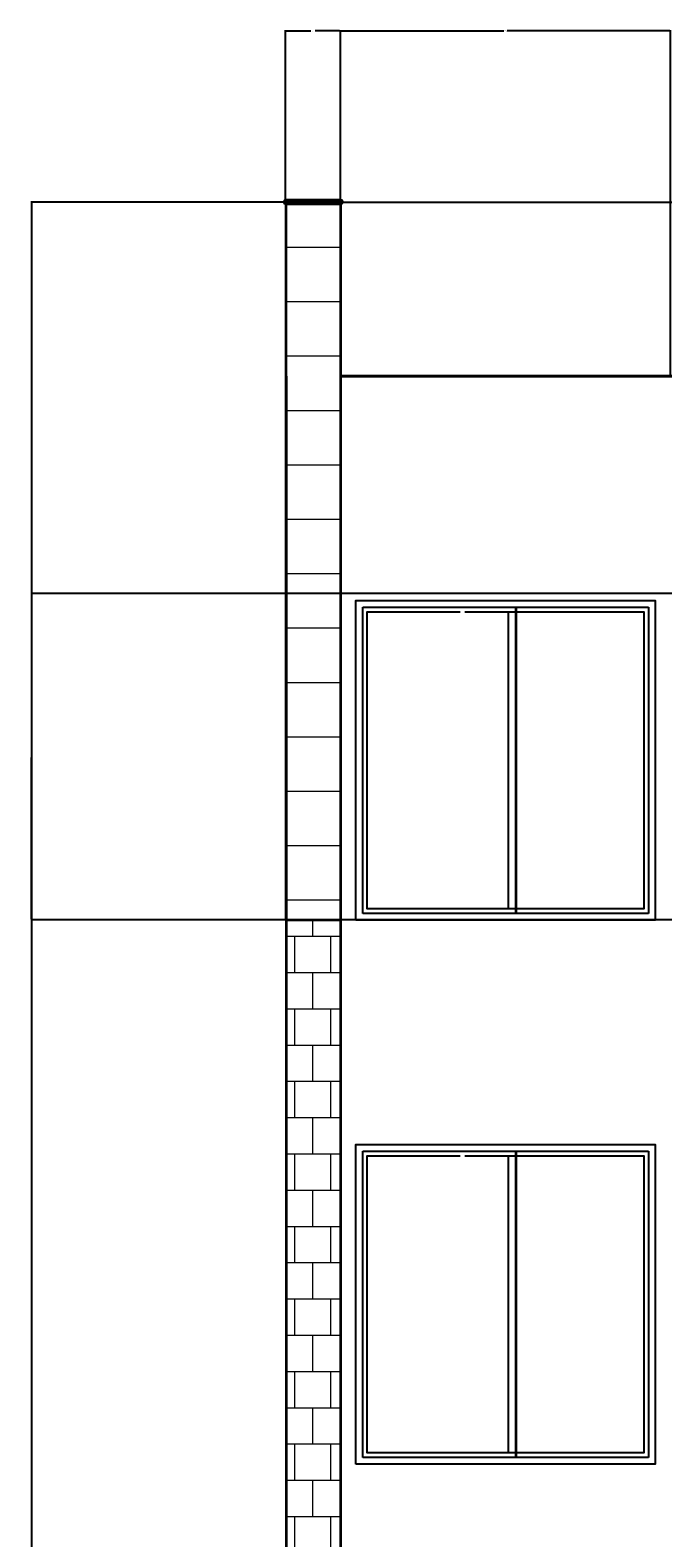
# Model space of a CAD drawing. Units: inches. Extents: x 10 to 404, y -77 to 696.
# Tile 4 of 5: x 10 to 149, y 363 to 696. Entities that reach past the tile are written whole.
import ezdxf

# ---------------------------------------------------------------- set-up
doc = ezdxf.new("R2010")
doc.units = ezdxf.units.IN
doc.header["$MEASUREMENT"] = 0
for name, color, linetype, lineweight in [('A-ANNO-DIMS', 2, 'Continuous', 18), ('A-ELEV', 7, 'Continuous', 35), ('A-ELEV-PATT', 8, 'Continuous', 13), ('A-GLAZ', 4, 'Continuous', 25)]:
    doc.layers.add(name, color=color, linetype=linetype, lineweight=lineweight)
doc.styles.get("Standard").update_dxf_attribs({"font": 'arial.ttf'})
doc.dimstyles.get("Standard").update_dxf_attribs({"dimtxt": 0.18, "dimasz": 0.18, "dimexe": 0.18, "dimexo": 0.0625, "dimgap": 0.09, "dimtad": 0, "dimtih": 1, "dimtoh": 1, "dimdec": 4, "dimzin": 0, "dimdsep": 46, "dimtxsty": 'Standard', "dimcen": 0.09, "dimadec": 0, "dimazin": 0, "dimtfac": 1, "dimtdec": 4, "dimtofl": 0, "dimtmove": 0, "dimatfit": 3, "dimfxl": 1, "dimtolj": 1, "dimtzin": 0, "dimarcsym": 0})

# ---------------------------------------------------------------- blocks, each defined once
blk = doc.blocks.new('WIN-SLIDING-2P')
for p, q in [((83.01, 21.05), (83.01, 88.58)), ((83.01, 88.58), (105.51, 88.58)), ((105.51, 88.58), (146.03, 88.58)), ((146.03, 88.58), (146.03, 21.05)), ((105.51, 21.05), (83.01, 21.05)), ((146.03, 21.05), (105.51, 21.05))]:
    blk.add_line(p, q)
blk.add_lwpolyline([(81.51, 19.55), (81.51, 90.08), (147.53, 90.08), (147.53, 19.55)], close=True)
blk.add_lwpolyline([(115.07, 87.58), (115.07, 22.05), (84.01, 22.05), (84.01, 87.58), (104.51, 87.58)])
blk = doc.blocks.new('*D10')
at = {"layer": 'A-ANNO-DIMS', "color": 0, "lineweight": -2, "transparency": 16777216}
for p, q in [((65.94, 657.96), (9.76, 657.96)), ((9.94, 657.78), (9.94, 315.77)), ((9.94, -26.6), (9.94, 315.41)), ((176.46, -26.78), (9.76, -26.78))]:
    blk.add_line(p, q, dxfattribs=at)
at = {"layer": 'A-ANNO-DIMS', "color": 0, "transparency": 16777216}
for points in [[(9.91, 657.78), (9.97, 657.78), (9.94, 657.96)], [(9.91, -26.6), (9.97, -26.6), (9.94, -26.78)]]:
    blk.add_solid(points, dxfattribs=at)
at = {"layer": 'Defpoints', "color": 0, "transparency": 16777216}
for p in [(9.94, 657.96), (66.01, 657.96), (176.53, -26.78)]:
    blk.add_point(p, dxfattribs=at)
at = {"layer": 'A-ANNO-DIMS', "color": 0, "transparency": 16777216, "insert": (9.94, 315.59), "char_height": 0.18, "attachment_point": 5}
blk.add_mtext('\\A1;684.7', dxfattribs=at)
blk = doc.blocks.new('*D17')
at = {"layer": 'A-ANNO-DIMS', "color": 0, "lineweight": -2, "transparency": 16777216}
for p, q in [((66.01, 658.02), (66.01, 695.87)), ((66.19, 695.69), (71.6, 695.69)), ((77.92, 695.69), (72.51, 695.69)), ((78.1, 657.66), (78.1, 695.87))]:
    blk.add_line(p, q, dxfattribs=at)
at = {"layer": 'A-ANNO-DIMS', "color": 0, "transparency": 16777216}
for points in [[(66.19, 695.72), (66.19, 695.66), (66.01, 695.69)], [(77.92, 695.72), (77.92, 695.66), (78.1, 695.69)]]:
    blk.add_solid(points, dxfattribs=at)
at = {"layer": 'Defpoints', "color": 0, "transparency": 16777216}
for p in [(78.1, 695.69), (66.01, 657.96), (78.1, 657.59)]:
    blk.add_point(p, dxfattribs=at)
at = {"layer": 'A-ANNO-DIMS', "color": 0, "transparency": 16777216, "insert": (72.05, 695.69), "char_height": 0.18, "attachment_point": 5}
blk.add_mtext('\\A1;12.095', dxfattribs=at)
blk = doc.blocks.new('*D18')
at = {"layer": 'A-ANNO-DIMS', "color": 0, "lineweight": -2, "transparency": 16777216}
for p, q in [((78.1, 619.62), (78.1, 695.87)), ((78.28, 695.69), (114.12, 695.69)), ((150.75, 695.69), (114.91, 695.69)), ((150.93, 619.62), (150.93, 695.87))]:
    blk.add_line(p, q, dxfattribs=at)
at = {"layer": 'A-ANNO-DIMS', "color": 0, "transparency": 16777216}
for points in [[(78.28, 695.72), (78.28, 695.66), (78.1, 695.69)], [(150.75, 695.72), (150.75, 695.66), (150.93, 695.69)]]:
    blk.add_solid(points, dxfattribs=at)
at = {"layer": 'Defpoints', "color": 0, "transparency": 16777216}
for p in [(150.93, 695.69), (78.1, 619.55), (150.93, 619.55)]:
    blk.add_point(p, dxfattribs=at)
at = {"layer": 'A-ANNO-DIMS', "color": 0, "transparency": 16777216, "insert": (114.52, 695.69), "char_height": 0.18, "attachment_point": 5}
blk.add_mtext('\\A1;72.83', dxfattribs=at)
blk = doc.blocks.new('*D35')
at = {"layer": 'A-ANNO-DIMS', "color": 0, "lineweight": -2, "transparency": 16777216}
for p, q in [((66.07, 657.96), (403.47, 657.96)), ((403.29, 657.78), (403.29, 638.94)), ((403.29, 619.73), (403.29, 638.58)), ((354.63, 619.55), (403.47, 619.55))]:
    blk.add_line(p, q, dxfattribs=at)
at = {"layer": 'A-ANNO-DIMS', "color": 0, "transparency": 16777216}
for points in [[(403.26, 657.78), (403.32, 657.78), (403.29, 657.96)], [(403.26, 619.73), (403.32, 619.73), (403.29, 619.55)]]:
    blk.add_solid(points, dxfattribs=at)
at = {"layer": 'Defpoints', "color": 0, "transparency": 16777216}
for p in [(66.01, 657.96), (403.29, 657.96), (354.56, 619.55)]:
    blk.add_point(p, dxfattribs=at)
at = {"layer": 'A-ANNO-DIMS', "color": 0, "transparency": 16777216, "insert": (403.29, 638.76), "char_height": 0.18, "attachment_point": 5}
blk.add_mtext('\\A1;38.41', dxfattribs=at)
blk = doc.blocks.new('*D71')
at = {"layer": 'A-ANNO-DIMS', "color": 0, "lineweight": -2, "transparency": 16777216}
for p, q in [((203.6, 571.6), (9.76, 571.6)), ((9.94, 571.42), (9.94, 535.78)), ((9.94, 499.78), (9.94, 535.42)), ((203.6, 499.6), (9.76, 499.6))]:
    blk.add_line(p, q, dxfattribs=at)
at = {"layer": 'A-ANNO-DIMS', "color": 0, "transparency": 16777216}
for points in [[(9.91, 571.42), (9.97, 571.42), (9.94, 571.6)], [(9.91, 499.78), (9.97, 499.78), (9.94, 499.6)]]:
    blk.add_solid(points, dxfattribs=at)
at = {"layer": 'Defpoints', "color": 0, "transparency": 16777216}
for p in [(9.94, 571.6), (203.67, 571.6), (203.67, 499.6)]:
    blk.add_point(p, dxfattribs=at)
at = {"layer": 'A-ANNO-DIMS', "color": 0, "transparency": 16777216, "insert": (9.94, 535.6), "char_height": 0.18, "attachment_point": 5}
blk.add_mtext('\\A1;72', dxfattribs=at)

msp = doc.modelspace()

# ---------------------------------------------------------------- hatches: boundary and pattern name
at = {"layer": 'A-ELEV-PATT'}
h = msp.add_hatch(dxfattribs=at)
h.set_pattern_fill('_USER', color=256, scale=12, pattern_type=0)
h.set_pattern_definition([(0, (0, 0), (0, 12), [])])
h.paths.add_polyline_path([(78.1013, 657.5934), (66.1013, 657.5934), (66.1013, 499.5535), (78.1013, 499.5535)])
h = msp.add_hatch(dxfattribs=at)
h.set_pattern_fill('AR-B88', color=256)
h.paths.add_polyline_path([(78.1013, 499.5535), (66.1013, 499.5535), (66.1013, 19.5535), (78.1013, 19.5535)])

# ---------------------------------------------------------------- linework, layer by layer
at = {"layer": 'A-ELEV'}
for p, q in [((78.1965, 658.3411), (66.0062, 658.3411)), ((66.1013, 619.5535), (66.1013, 19.5535)), ((341.8668, 619.5535), (78.1013, 619.5535)), ((78.1013, 619.5535), (341.8668, 619.5535)), ((78.1013, 619.5535), (78.1013, 19.5535)), ((116.8527, 501.0535), (116.8527, 568.5811)), ((116.8527, 381.0535), (116.8527, 448.5811))]:
    msp.add_line(p, q, dxfattribs=at)
msp.add_lwpolyline([(78.1013, 499.5535), (66.1013, 499.5535), (66.1013, 657.5934), (78.1013, 657.5934)], close=True, dxfattribs=at)
for centre, start, end in [((66.0062, 657.9612), 90, 284.503141), ((78.1965, 657.9612), 255.496859, 90)]:
    msp.add_arc(centre, 0.3799, start, end, dxfattribs=at)
at = {"layer": 'A-GLAZ'}
for points in [[(105.5054, 567.5811), (145.0304, 567.5811), (145.0304, 502.0535), (105.5054, 502.0535)], [(105.5054, 447.5811), (145.0304, 447.5811), (145.0304, 382.0535), (105.5054, 382.0535)]]:
    msp.add_lwpolyline(points, dxfattribs=at)

# ---------------------------------------------------------------- block references
for p in [(0, 480), (0, 360)]:
    msp.add_blockref('WIN-SLIDING-2P', p, dxfattribs=at)

# ---------------------------------------------------------------- dimensions: what is measured, and where the dimension line sits
at = {"layer": 'A-ANNO-DIMS'}
for base, p1, p2, override, picture, middle in [((78.1013, 695.6911), (66.0062, 657.9612), (78.1013, 657.5934), {"dimdec": 3, "dimlfac": 1, "dimrnd": 0, "dimzin": 0, "dimdsep": 46, "dimlunit": 2}, '*D17', (72.0538, 695.6911)), ((150.9344, 695.6911), (78.1013, 619.5535), (150.9344, 619.5535), {"dimdec": 2, "dimlfac": 1, "dimrnd": 0, "dimzin": 0, "dimdsep": 46, "dimlunit": 2}, '*D18', (114.5179, 695.6911))]:
    dim = msp.add_linear_dim(base=base, p1=p1, p2=p2, dimstyle='Standard', override=override, dxfattribs=at)
    dim.commit()
    dim.dimension.update_dxf_attribs({"geometry": picture, "text_midpoint": middle})
for base, p1, p2, override, picture, middle in [((9.9405, 657.9612), (176.5266, -26.7816), (66.0062, 657.9612), {"dimdec": 1, "dimlfac": 1, "dimrnd": 0, "dimzin": 0, "dimdsep": 46, "dimlunit": 2}, '*D10', (9.9405, 315.5898)), ((403.2856, 657.9612), (354.5631, 619.5535), (66.0062, 657.9612), {"dimdec": 2, "dimlfac": 1, "dimrnd": 0, "dimzin": 0, "dimdsep": 46, "dimlunit": 2}, '*D35', (403.2856, 638.7574)), ((9.9405, 571.6046), (203.6671, 499.6046), (203.6671, 571.6046), {"dimdec": 0, "dimlfac": 1, "dimrnd": 0, "dimzin": 0, "dimdsep": 46, "dimlunit": 2}, '*D71', (9.9405, 535.6046))]:
    dim = msp.add_linear_dim(base=base, p1=p1, p2=p2, angle=90, dimstyle='Standard', override=override, dxfattribs=at)
    dim.commit()
    dim.dimension.update_dxf_attribs({"geometry": picture, "text_midpoint": middle})

doc.saveas('drawing.dxf')
